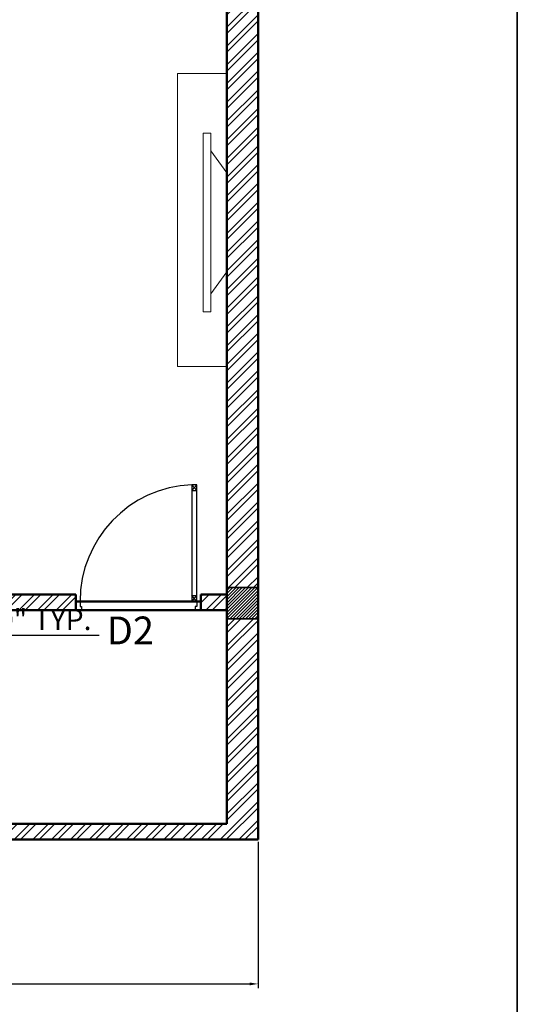
# Model space of a CAD drawing. Units: millimetres. Extents: x 20768 to 23556, y 50760 to 52704.
# Tile 19 of 36: x 21491 to 21634, y 51783 to 52066. Entities that reach past the tile are written whole.
import ezdxf

# ---------------------------------------------------------------- set-up
doc = ezdxf.new("R2010")
doc.units = ezdxf.units.MM
for name, color, linetype, lineweight in [('A-ANNO-TTLB', 7, 'Continuous', 35), ('A-AREA-IDEN', 40, 'Continuous', 18), ('A-DOOR', 3, 'Continuous', 25), ('A-FURN', 8, 'Continuous', 18), ('A-WALL', 7, 'Continuous', 50), ('A-WALL-PATT', 8, 'Continuous', 13), ('S-ANNO-DIMS', 2, 'Continuous', 18), ('S-COLS', 20, 'Continuous', 35)]:
    doc.layers.add(name, color=color, linetype=linetype, lineweight=lineweight)
doc.styles.get("Standard").update_dxf_attribs({"font": 'arial.ttf'})
doc.dimstyles.new('ISO-25', dxfattribs={"dimtxt": 6, "dimasz": 2.5, "dimexe": 1.25, "dimexo": 0.625, "dimtad": 1, "dimdec": 0, "dimlunit": 3, "dimtxsty": 'Standard', "dimcen": 2.5, "dimadec": 0, "dimazin": 0, "dimtfac": 1, "dimtdec": 0, "dimtmove": 0, "dimatfit": 3, "dimfxl": 1, "dimarcsym": 0})
pattern_1 = [(45, (-37.4434, 0), (-2.69407684, 2.69407684), []), (45, (-35.6473, 0), (-2.69407684, 2.69407684), [])]

# ---------------------------------------------------------------- blocks, each defined once
blk = doc.blocks.new('Puerta 01')
for p, q in [((-0.7745, -0.0264), (-0.7368, -0.0584)), ((-0.7745, -0.0584), (-0.7368, -0.0264)), ((-0.7368, -0.0584), (-0.7368, -0.0264)), ((-0.028, -0.0584), (-0.0657, -0.0264)), ((-0.028, -0.0264), (-0.0657, -0.0584)), ((-0.0657, -0.0584), (-0.0657, -0.0264))]:
    blk.add_line(p, q)
for points in [[(-0.028, 0), (-0.028, -0.0264), (0.004, -0.0264), (0.004, -0.036), (0.028, -0.036), (0.028, 0)], [(-0.028, -0.0264), (-0.7745, -0.0264), (-0.7745, -0.0584), (-0.028, -0.0584)], [(0.004, -0.7736), (0.004, -0.764), (0.028, -0.764), (0.028, -0.8), (-0.028, -0.8), (-0.028, -0.7736)]]:
    blk.add_lwpolyline(points, close=True)
blk.add_arc((-0.028, -0.0264), 0.7472, 182.45453, 270)
blk = doc.blocks.new('tv')
for p, q in [((20989.25, 52437.95), (20993.93, 52444.3)), ((20989.25, 52409.51), (20993.93, 52403.15))]:
    blk.add_line(p, q)
for points in [[(20989.25, 52466.51), (21003.46, 52466.51), (21003.46, 52382.21), (20989.25, 52382.21)], [(20993.93, 52449.42), (20996.05, 52449.42), (20996.05, 52398.03), (20993.93, 52398.03)]]:
    blk.add_lwpolyline(points, close=True)
blk = doc.blocks.new('COL-PLAN')
blk.add_line((0, 9), (9, 9))
blk.add_lwpolyline([(9, 9), (0, 9), (0, 0), (9, 0)], close=True)
blk = doc.blocks.new('*D179')
at = {"layer": 'Defpoints', "color": 0, "transparency": 16777216}
for p in [(21386.24, 51895.9), (21434.24, 51895.9), (21434.24, 51888.7)]:
    blk.add_point(p, dxfattribs=at)
at = {"layer": 'S-ANNO-DIMS', "color": 0, "lineweight": -2, "transparency": 16777216}
for p, q in [((21386.24, 51895.27), (21386.24, 51887.45)), ((21434.24, 51895.27), (21434.24, 51887.45)), ((21388.74, 51888.7), (21431.74, 51888.7)), ((21434.24, 51888.7), (21513.92, 51888.7))]:
    blk.add_line(p, q, dxfattribs=at)
at = {"layer": 'S-ANNO-DIMS', "color": 0, "transparency": 16777216}
for points in [[(21388.74, 51889.11), (21388.74, 51888.28), (21386.24, 51888.7)], [(21431.74, 51889.11), (21431.74, 51888.28), (21434.24, 51888.7)]]:
    blk.add_solid(points, dxfattribs=at)
at = {"layer": 'S-ANNO-DIMS', "color": 0, "transparency": 16777216, "insert": (21475.33, 51892.43), "char_height": 6, "attachment_point": 5}
blk.add_mtext('WINDOW 4\'-0" TYP.', dxfattribs=at)
blk = doc.blocks.new('*D210')
at = {"layer": 'Defpoints', "color": 0, "transparency": 16777216}
for p in [(21325.74, 51829.9), (21559.74, 51829.9), (21559.74, 51788.4)]:
    blk.add_point(p, dxfattribs=at)
at = {"layer": 'S-ANNO-DIMS', "color": 0, "lineweight": -2, "transparency": 16777216}
for p, q in [((21325.74, 51829.27), (21325.74, 51787.15)), ((21559.74, 51829.27), (21559.74, 51787.15)), ((21328.24, 51788.4), (21557.24, 51788.4))]:
    blk.add_line(p, q, dxfattribs=at)
at = {"layer": 'S-ANNO-DIMS', "color": 0, "transparency": 16777216}
for points in [[(21328.24, 51788.81), (21328.24, 51787.98), (21325.74, 51788.4)], [(21557.24, 51788.81), (21557.24, 51787.98), (21559.74, 51788.4)]]:
    blk.add_solid(points, dxfattribs=at)
at = {"layer": 'S-ANNO-DIMS', "color": 0, "transparency": 16777216, "insert": (21442.74, 51792.09), "char_height": 6, "attachment_point": 5}
blk.add_mtext('19\'-6"', dxfattribs=at)

msp = doc.modelspace()

# ---------------------------------------------------------------- hatches: boundary and pattern name
at = {"layer": 'A-WALL-PATT'}
h = msp.add_hatch(dxfattribs=at)
h.set_pattern_fill('ANSI32', color=256, scale=0.4)
h.set_pattern_definition(pattern_1)
h.paths.add_polyline_path([(21559.74, 52078.62), (21550.74, 52078.62), (21550.74, 51902.4), (21559.74, 51902.4)])
h = msp.add_hatch(dxfattribs=at)
h.set_pattern_fill('ANSI31', color=256, scale=0.2)
h.set_pattern_definition([(45, (345.4904, 0), (-0.449012806, 0.449012806), [])])
h.paths.add_polyline_path([(21559.74, 51902.4), (21550.74, 51902.4), (21550.74, 51893.4), (21559.74, 51893.4)])
h = msp.add_hatch(dxfattribs=at)
h.set_pattern_fill('ANSI32', color=256, scale=0.4)
h.set_pattern_definition(pattern_1)
h.paths.add_polyline_path([(21507.24, 51898.42), (21507.24, 51900.4), (21434.24, 51900.4), (21434.24, 51895.9), (21507.24, 51895.9)])
h = msp.add_hatch(dxfattribs=at)
h.set_pattern_fill('ANSI32', color=256, scale=0.4)
h.set_pattern_definition(pattern_1)
h.paths.add_polyline_path([(21550.74, 51900.4), (21543.24, 51900.4), (21543.24, 51895.9), (21550.74, 51895.9)])
h = msp.add_hatch(dxfattribs=at)
h.set_pattern_fill('ANSI32', color=256, scale=0.4)
h.set_pattern_definition(pattern_1)
h.paths.add_polyline_path([(21559.74, 51893.4), (21550.74, 51893.4), (21550.74, 51834.4), (21334.74, 51834.4), (21334.74, 51829.9), (21559.74, 51829.9)])

# ---------------------------------------------------------------- linework, layer by layer
at = {"layer": 'A-ANNO-TTLB'}
msp.add_line((21634.36, 52703.98), (21634.36, 51623.53), dxfattribs=at)
at = {"layer": 'A-WALL'}
for p, q in [((21559.74, 52522.9), (21559.74, 51829.9)), ((21550.74, 52513.9), (21550.74, 51834.4)), ((21334.74, 51900.4), (21507.24, 51900.4)), ((21507.24, 51900.4), (21507.24, 51895.9)), ((21543.24, 51900.4), (21543.24, 51895.9)), ((21543.24, 51900.4), (21550.74, 51900.4)), ((21334.74, 51895.9), (21507.24, 51895.9)), ((21507.24, 51898.42), (21543.24, 51898.42)), ((21507.24, 51895.9), (21543.24, 51895.9)), ((21543.24, 51895.9), (21550.74, 51895.9)), ((21325.74, 51834.4), (21550.74, 51834.4)), ((21325.74, 51829.9), (21559.74, 51829.9))]:
    msp.add_line(p, q, dxfattribs=at)

# ---------------------------------------------------------------- block references
at = {"layer": 'A-DOOR', "xscale": 45.00000000000065, "yscale": 45.00000000000065, "zscale": 45.00000000000065, "rotation": 270.0000000000003}
msp.add_blockref('Puerta 01', (21543.24, 51897.16), dxfattribs=at)
at = {"layer": 'A-FURN', "xscale": -1}
msp.add_blockref('tv', (42539.99, -416.25), dxfattribs=at)
at = {"layer": 'S-COLS'}
msp.add_blockref('COL-PLAN', (21550.74, 51893.4), dxfattribs=at)

# ---------------------------------------------------------------- texts
at = {"layer": 'A-AREA-IDEN', "insert": (21513.71, 51894.08), "char_height": 8, "attachment_point": 1}
msp.add_mtext_dynamic_manual_height_columns(' D2', width=27.5349, gutter_width=12.5, heights=[0], dxfattribs=at)

# ---------------------------------------------------------------- dimensions: what is measured, and where the dimension line sits
at = {"layer": 'S-ANNO-DIMS'}
dim = msp.add_linear_dim(base=(21434.24, 51888.7), p1=(21386.24, 51895.9), p2=(21434.24, 51895.9), text='WINDOW <> TYP.', dimstyle='ISO-25', override={"dimdec": 1, "dimrnd": 0, "dimzin": 1, "dimlunit": 4, "dimfrac": 2}, dxfattribs=at)
dim.commit()
dim.dimension.update_dxf_attribs({"geometry": '*D179', "text_midpoint": (21475.33, 51892.43)})
dim = msp.add_linear_dim(base=(21559.74, 51788.4), p1=(21325.74, 51829.9), p2=(21559.74, 51829.9), dimstyle='ISO-25', override={"dimdec": 1, "dimlfac": 1, "dimrnd": 0, "dimzin": 1, "dimdsep": 46, "dimlunit": 4, "dimfrac": 2}, dxfattribs=at)
dim.commit()
dim.dimension.update_dxf_attribs({"geometry": '*D210', "text_midpoint": (21442.74, 51792.09)})

doc.saveas('drawing.dxf')
